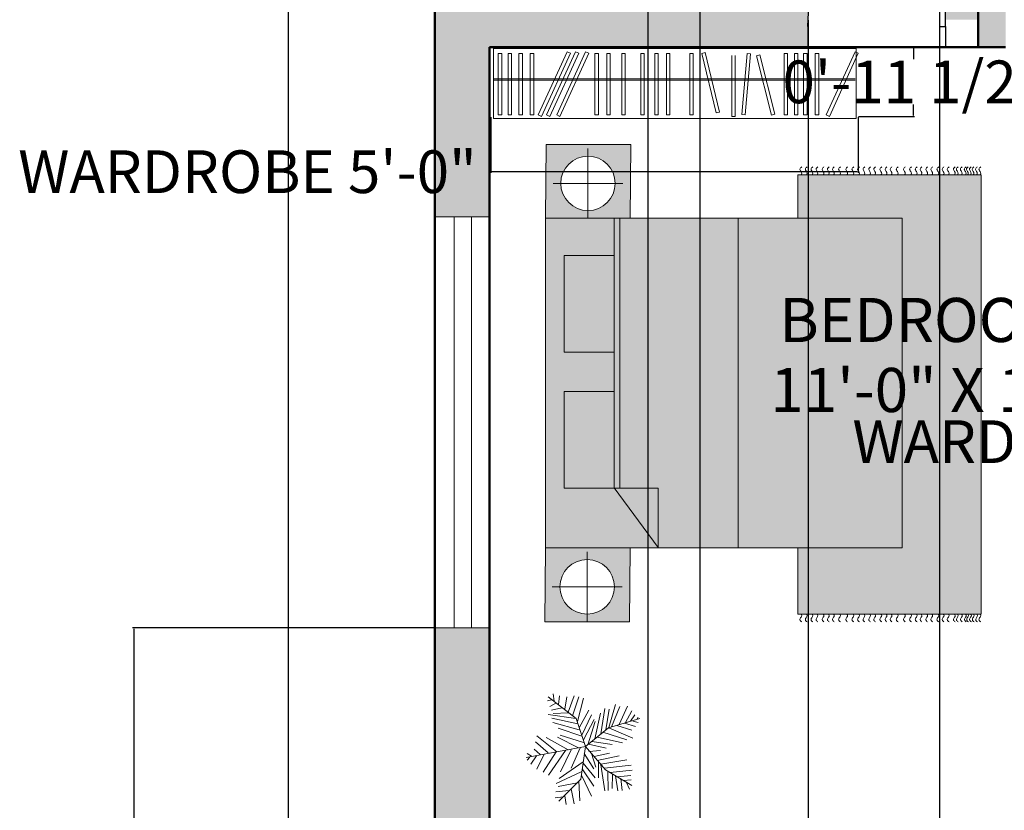
# Model space of a CAD drawing. Units: inches. Extents: x 2974 to 3443, y 2405 to 2963.
# Tile 10 of 13: x 2974 to 3136, y 2711 to 2840. Entities that reach past the tile are written whole.
import ezdxf

# ---------------------------------------------------------------- set-up
doc = ezdxf.new("R2010")
doc.units = ezdxf.units.IN
doc.header["$MEASUREMENT"] = 0
doc.layers.get('0').update_dxf_attribs({"color": 251})
for name, color, linetype, lineweight in [('A-ANNO-DIMS', 2, 'Continuous', 18), ('A-AREA-IDEN', 250, 'Continuous', 25), ('A-DOOR', 32, 'Continuous', 25), ('A-FLOR-PATT', 9, 'Continuous', 13), ('A-WALL-PATT', 252, 'Continuous', 13), ('closet', 32, 'Continuous', 20), ('furniture', 32, 'Continuous', 18), ('greenary', 106, 'Continuous', 13), ('walls', 250, 'Continuous', 50), ('windows', 159, 'Continuous', 20)]:
    doc.layers.add(name, color=color, linetype=linetype, lineweight=lineweight)
doc.layers.add('A-FURN-PATT', color=254, linetype='Continuous', lineweight=13, true_color=0xfeeab9)
doc.styles.get("Standard").update_dxf_attribs({"font": 'arial.ttf'})
doc.dimstyles.get("Standard").update_dxf_attribs({"dimtxt": 7, "dimasz": 0.18, "dimexe": 0.18, "dimexo": 0.0625, "dimgap": 0.09, "dimtad": 0, "dimtih": 1, "dimtoh": 1, "dimzin": 0, "dimdsep": 46, "dimlunit": 3, "dimtxsty": 'Standard', "dimcen": 0.09, "dimadec": 0, "dimazin": 0, "dimtfac": 1, "dimtofl": 0, "dimtmove": 0, "dimatfit": 3, "dimfxl": 1, "dimtolj": 1, "dimtzin": 0, "dimarcsym": 0})

# ---------------------------------------------------------------- blocks, each defined once
blk = doc.blocks.new('*U2')
for p, q in [((0, 0), (0, -6)), ((40, 0), (40, -6))]:
    blk.add_line(p, q)
blk.add_lwpolyline([(0, 0), (0, 40), (1.75, 40), (1.75, 0)], close=True)
blk.add_arc((0, 0), 40, 0, 90)
blk = doc.blocks.new('CARPET')
at = {"layer": 'furniture'}
for p, q in [((-51.53, -98.11), (-51.53, -55.12)), ((-51.53, -55.12), (-41.27, -55.12)), ((36, -55.12), (51.55, -55.12)), ((51.55, -55.12), (51.55, -98.11)), ((51.55, -98.11), (-51.53, -98.11))]:
    blk.add_line(p, q, dxfattribs=at)
for points, knots in [([(-53.37, -55.99), (-53.22, -55.8), (-52.9, -55.41), (-52.34, -55.8), (-51.89, -56.08), (-51.65, -55.91), (-51.53, -55.83)], [0, 0, 0, 0, 0.653278, 1.290138, 1.740457, 2.114451, 2.114451, 2.114451, 2.114451]), ([(-53.37, -57.26), (-53.22, -57.07), (-52.9, -56.67), (-52.34, -57.07), (-51.89, -57.35), (-51.65, -57.17), (-51.53, -57.1)], [0, 0, 0, 0, 0.653278, 1.290138, 1.740457, 2.114451, 2.114451, 2.114451, 2.114451]), ([(53.37, -55.99), (53.22, -55.8), (52.9, -55.41), (52.34, -55.8), (51.89, -56.08), (51.65, -55.91), (51.53, -55.83)], [0, 0, 0, 0, 0.653278, 1.290138, 1.740457, 2.114451, 2.114451, 2.114451, 2.114451]), ([(53.37, -57.26), (53.22, -57.07), (52.9, -56.67), (52.34, -57.07), (51.89, -57.35), (51.65, -57.17), (51.53, -57.1)], [0, 0, 0, 0, 0.653278, 1.290138, 1.740457, 2.114451, 2.114451, 2.114451, 2.114451]), ([(-53.37, -58.59), (-53.22, -58.4), (-52.9, -58.01), (-52.34, -58.4), (-51.89, -58.68), (-51.65, -58.5), (-51.53, -58.43)], [0, 0, 0, 0, 0.653278, 1.290138, 1.740457, 2.114451, 2.114451, 2.114451, 2.114451]), ([(-53.37, -59.78), (-53.22, -59.58), (-52.9, -59.19), (-52.34, -59.58), (-51.89, -59.86), (-51.65, -59.69), (-51.53, -59.61)], [0, 0, 0, 0, 0.653278, 1.290138, 1.740457, 2.114451, 2.114451, 2.114451, 2.114451]), ([(53.37, -58.59), (53.22, -58.4), (52.9, -58.01), (52.34, -58.4), (51.89, -58.68), (51.65, -58.5), (51.53, -58.43)], [0, 0, 0, 0, 0.653278, 1.290138, 1.740457, 2.114451, 2.114451, 2.114451, 2.114451]), ([(53.37, -59.78), (53.22, -59.58), (52.9, -59.19), (52.34, -59.58), (51.89, -59.86), (51.65, -59.69), (51.53, -59.61)], [0, 0, 0, 0, 0.653278, 1.290138, 1.740457, 2.114451, 2.114451, 2.114451, 2.114451]), ([(-53.37, -61.22), (-53.22, -61.02), (-52.9, -60.63), (-52.34, -61.02), (-51.89, -61.3), (-51.65, -61.13), (-51.53, -61.05)], [0, 0, 0, 0, 0.653278, 1.290138, 1.740457, 2.114451, 2.114451, 2.114451, 2.114451]), ([(-53.37, -62.44), (-53.22, -62.25), (-52.9, -61.86), (-52.34, -62.25), (-51.89, -62.53), (-51.65, -62.36), (-51.53, -62.28)], [0, 0, 0, 0, 0.653278, 1.290138, 1.740457, 2.114451, 2.114451, 2.114451, 2.114451]), ([(53.37, -61.22), (53.22, -61.02), (52.9, -60.63), (52.34, -61.02), (51.89, -61.3), (51.65, -61.13), (51.53, -61.05)], [0, 0, 0, 0, 0.653278, 1.290138, 1.740457, 2.114451, 2.114451, 2.114451, 2.114451]), ([(53.37, -62.44), (53.22, -62.25), (52.9, -61.86), (52.34, -62.25), (51.89, -62.53), (51.65, -62.36), (51.53, -62.28)], [0, 0, 0, 0, 0.653278, 1.290138, 1.740457, 2.114451, 2.114451, 2.114451, 2.114451]), ([(-53.37, -63.63), (-53.22, -63.43), (-52.9, -63.04), (-52.34, -63.43), (-51.89, -63.72), (-51.65, -63.54), (-51.53, -63.46)], [0, 0, 0, 0, 0.653278, 1.290138, 1.740457, 2.114451, 2.114451, 2.114451, 2.114451]), ([(-53.37, -65.07), (-53.22, -64.87), (-52.9, -64.48), (-52.34, -64.87), (-51.89, -65.15), (-51.65, -64.98), (-51.53, -64.9)], [0, 0, 0, 0, 0.653278, 1.290138, 1.740457, 2.114451, 2.114451, 2.114451, 2.114451]), ([(53.37, -63.63), (53.22, -63.43), (52.9, -63.04), (52.34, -63.43), (51.89, -63.72), (51.65, -63.54), (51.53, -63.46)], [0, 0, 0, 0, 0.653278, 1.290138, 1.740457, 2.114451, 2.114451, 2.114451, 2.114451]), ([(53.37, -65.07), (53.22, -64.87), (52.9, -64.48), (52.34, -64.87), (51.89, -65.15), (51.65, -64.98), (51.53, -64.9)], [0, 0, 0, 0, 0.653278, 1.290138, 1.740457, 2.114451, 2.114451, 2.114451, 2.114451]), ([(-53.37, -66.76), (-53.22, -66.56), (-52.9, -66.17), (-52.34, -66.56), (-51.89, -66.84), (-51.65, -66.67), (-51.53, -66.59)], [0, 0, 0, 0, 0.653278, 1.290138, 1.740457, 2.114451, 2.114451, 2.114451, 2.114451]), ([(53.37, -66.76), (53.22, -66.56), (52.9, -66.17), (52.34, -66.56), (51.89, -66.84), (51.65, -66.67), (51.53, -66.59)], [0, 0, 0, 0, 0.653278, 1.290138, 1.740457, 2.114451, 2.114451, 2.114451, 2.114451]), ([(-53.37, -68.2), (-53.22, -68), (-52.9, -67.61), (-52.34, -68), (-51.89, -68.28), (-51.65, -68.11), (-51.53, -68.03)], [0, 0, 0, 0, 0.653278, 1.290138, 1.740457, 2.114451, 2.114451, 2.114451, 2.114451]), ([(-53.37, -69.53), (-53.22, -69.33), (-52.9, -68.94), (-52.34, -69.33), (-51.89, -69.61), (-51.65, -69.44), (-51.53, -69.36)], [0, 0, 0, 0, 0.653278, 1.290138, 1.740457, 2.114451, 2.114451, 2.114451, 2.114451]), ([(53.37, -68.2), (53.22, -68), (52.9, -67.61), (52.34, -68), (51.89, -68.28), (51.65, -68.11), (51.53, -68.03)], [0, 0, 0, 0, 0.653278, 1.290138, 1.740457, 2.114451, 2.114451, 2.114451, 2.114451]), ([(53.37, -69.53), (53.22, -69.33), (52.9, -68.94), (52.34, -69.33), (51.89, -69.61), (51.65, -69.44), (51.53, -69.36)], [0, 0, 0, 0, 0.653278, 1.290138, 1.740457, 2.114451, 2.114451, 2.114451, 2.114451]), ([(-53.37, -70.79), (-53.22, -70.6), (-52.9, -70.21), (-52.34, -70.6), (-51.89, -70.88), (-51.65, -70.7), (-51.53, -70.63)], [0, 0, 0, 0, 0.653278, 1.290138, 1.740457, 2.114451, 2.114451, 2.114451, 2.114451]), ([(53.37, -70.79), (53.22, -70.6), (52.9, -70.21), (52.34, -70.6), (51.89, -70.88), (51.65, -70.7), (51.53, -70.63)], [0, 0, 0, 0, 0.653278, 1.290138, 1.740457, 2.114451, 2.114451, 2.114451, 2.114451]), ([(-53.37, -72.12), (-53.22, -71.93), (-52.9, -71.54), (-52.34, -71.93), (-51.89, -72.21), (-51.65, -72.04), (-51.53, -71.96)], [0, 0, 0, 0, 0.653278, 1.290138, 1.740457, 2.114451, 2.114451, 2.114451, 2.114451]), ([(-53.37, -73.31), (-53.22, -73.11), (-52.9, -72.72), (-52.34, -73.11), (-51.89, -73.4), (-51.65, -73.22), (-51.53, -73.14)], [0, 0, 0, 0, 0.653278, 1.290138, 1.740457, 2.114451, 2.114451, 2.114451, 2.114451]), ([(53.37, -72.12), (53.22, -71.93), (52.9, -71.54), (52.34, -71.93), (51.89, -72.21), (51.65, -72.04), (51.53, -71.96)], [0, 0, 0, 0, 0.653278, 1.290138, 1.740457, 2.114451, 2.114451, 2.114451, 2.114451]), ([(53.37, -73.31), (53.22, -73.11), (52.9, -72.72), (52.34, -73.11), (51.89, -73.4), (51.65, -73.22), (51.53, -73.14)], [0, 0, 0, 0, 0.653278, 1.290138, 1.740457, 2.114451, 2.114451, 2.114451, 2.114451]), ([(-53.37, -74.75), (-53.22, -74.55), (-52.9, -74.16), (-52.34, -74.55), (-51.89, -74.83), (-51.65, -74.66), (-51.53, -74.58)], [0, 0, 0, 0, 0.653278, 1.290138, 1.740457, 2.114451, 2.114451, 2.114451, 2.114451]), ([(-53.37, -75.98), (-53.22, -75.78), (-52.9, -75.39), (-52.34, -75.78), (-51.89, -76.06), (-51.65, -75.89), (-51.53, -75.81)], [0, 0, 0, 0, 0.653278, 1.290138, 1.740457, 2.114451, 2.114451, 2.114451, 2.114451]), ([(53.37, -74.75), (53.22, -74.55), (52.9, -74.16), (52.34, -74.55), (51.89, -74.83), (51.65, -74.66), (51.53, -74.58)], [0, 0, 0, 0, 0.653278, 1.290138, 1.740457, 2.114451, 2.114451, 2.114451, 2.114451]), ([(53.37, -75.98), (53.22, -75.78), (52.9, -75.39), (52.34, -75.78), (51.89, -76.06), (51.65, -75.89), (51.53, -75.81)], [0, 0, 0, 0, 0.653278, 1.290138, 1.740457, 2.114451, 2.114451, 2.114451, 2.114451]), ([(-53.37, -77.16), (-53.22, -76.96), (-52.9, -76.57), (-52.34, -76.96), (-51.89, -77.25), (-51.65, -77.07), (-51.53, -76.99)], [0, 0, 0, 0, 0.653278, 1.290138, 1.740457, 2.114451, 2.114451, 2.114451, 2.114451]), ([(-53.37, -78.6), (-53.22, -78.4), (-52.9, -78.01), (-52.34, -78.4), (-51.89, -78.68), (-51.65, -78.51), (-51.53, -78.43)], [0, 0, 0, 0, 0.653278, 1.290138, 1.740457, 2.114451, 2.114451, 2.114451, 2.114451]), ([(53.37, -77.16), (53.22, -76.96), (52.9, -76.57), (52.34, -76.96), (51.89, -77.25), (51.65, -77.07), (51.53, -76.99)], [0, 0, 0, 0, 0.653278, 1.290138, 1.740457, 2.114451, 2.114451, 2.114451, 2.114451]), ([(53.37, -78.6), (53.22, -78.4), (52.9, -78.01), (52.34, -78.4), (51.89, -78.68), (51.65, -78.51), (51.53, -78.43)], [0, 0, 0, 0, 0.653278, 1.290138, 1.740457, 2.114451, 2.114451, 2.114451, 2.114451]), ([(-53.37, -80.29), (-53.22, -80.09), (-52.9, -79.7), (-52.34, -80.09), (-51.89, -80.37), (-51.65, -80.2), (-51.53, -80.12)], [0, 0, 0, 0, 0.653278, 1.290138, 1.740457, 2.114451, 2.114451, 2.114451, 2.114451]), ([(53.37, -80.29), (53.22, -80.09), (52.9, -79.7), (52.34, -80.09), (51.89, -80.37), (51.65, -80.2), (51.53, -80.12)], [0, 0, 0, 0, 0.653278, 1.290138, 1.740457, 2.114451, 2.114451, 2.114451, 2.114451]), ([(-53.37, -81.73), (-53.22, -81.53), (-52.9, -81.14), (-52.34, -81.53), (-51.89, -81.81), (-51.65, -81.64), (-51.53, -81.56)], [0, 0, 0, 0, 0.653278, 1.290138, 1.740457, 2.114451, 2.114451, 2.114451, 2.114451]), ([(-53.37, -83.06), (-53.22, -82.86), (-52.9, -82.47), (-52.34, -82.86), (-51.89, -83.14), (-51.65, -82.97), (-51.53, -82.89)], [0, 0, 0, 0, 0.653278, 1.290138, 1.740457, 2.114451, 2.114451, 2.114451, 2.114451]), ([(53.37, -81.73), (53.22, -81.53), (52.9, -81.14), (52.34, -81.53), (51.89, -81.81), (51.65, -81.64), (51.53, -81.56)], [0, 0, 0, 0, 0.653278, 1.290138, 1.740457, 2.114451, 2.114451, 2.114451, 2.114451]), ([(53.37, -83.06), (53.22, -82.86), (52.9, -82.47), (52.34, -82.86), (51.89, -83.14), (51.65, -82.97), (51.53, -82.89)], [0, 0, 0, 0, 0.653278, 1.290138, 1.740457, 2.114451, 2.114451, 2.114451, 2.114451]), ([(-53.37, -84.18), (-53.22, -83.99), (-52.9, -83.6), (-52.34, -83.99), (-51.89, -84.27), (-51.65, -84.09), (-51.53, -84.02)], [0, 0, 0, 0, 0.653278, 1.290138, 1.740457, 2.114451, 2.114451, 2.114451, 2.114451]), ([(-53.37, -85.51), (-53.22, -85.32), (-52.9, -84.93), (-52.34, -85.32), (-51.89, -85.6), (-51.65, -85.42), (-51.53, -85.35)], [0, 0, 0, 0, 0.653278, 1.290138, 1.740457, 2.114451, 2.114451, 2.114451, 2.114451]), ([(53.37, -84.18), (53.22, -83.99), (52.9, -83.6), (52.34, -83.99), (51.89, -84.27), (51.65, -84.09), (51.53, -84.02)], [0, 0, 0, 0, 0.653278, 1.290138, 1.740457, 2.114451, 2.114451, 2.114451, 2.114451]), ([(53.37, -85.51), (53.22, -85.32), (52.9, -84.93), (52.34, -85.32), (51.89, -85.6), (51.65, -85.42), (51.53, -85.35)], [0, 0, 0, 0, 0.653278, 1.290138, 1.740457, 2.114451, 2.114451, 2.114451, 2.114451]), ([(-53.37, -86.7), (-53.22, -86.5), (-52.9, -86.11), (-52.34, -86.5), (-51.89, -86.78), (-51.65, -86.61), (-51.53, -86.53)], [0, 0, 0, 0, 0.653278, 1.290138, 1.740457, 2.114451, 2.114451, 2.114451, 2.114451]), ([(-53.37, -88.14), (-53.22, -87.94), (-52.9, -87.55), (-52.34, -87.94), (-51.89, -88.22), (-51.65, -88.05), (-51.53, -87.97)], [0, 0, 0, 0, 0.653278, 1.290138, 1.740457, 2.114451, 2.114451, 2.114451, 2.114451]), ([(53.37, -86.7), (53.22, -86.5), (52.9, -86.11), (52.34, -86.5), (51.89, -86.78), (51.65, -86.61), (51.53, -86.53)], [0, 0, 0, 0, 0.653278, 1.290138, 1.740457, 2.114451, 2.114451, 2.114451, 2.114451]), ([(53.37, -88.14), (53.22, -87.94), (52.9, -87.55), (52.34, -87.94), (51.89, -88.22), (51.65, -88.05), (51.53, -87.97)], [0, 0, 0, 0, 0.653278, 1.290138, 1.740457, 2.114451, 2.114451, 2.114451, 2.114451]), ([(-53.37, -89.36), (-53.22, -89.17), (-52.9, -88.78), (-52.34, -89.17), (-51.89, -89.45), (-51.65, -89.28), (-51.53, -89.2)], [0, 0, 0, 0, 0.653278, 1.290138, 1.740457, 2.114451, 2.114451, 2.114451, 2.114451]), ([(53.37, -89.36), (53.22, -89.17), (52.9, -88.78), (52.34, -89.17), (51.89, -89.45), (51.65, -89.28), (51.53, -89.2)], [0, 0, 0, 0, 0.653278, 1.290138, 1.740457, 2.114451, 2.114451, 2.114451, 2.114451]), ([(-53.37, -90.55), (-53.22, -90.35), (-52.9, -89.96), (-52.34, -90.35), (-51.89, -90.64), (-51.65, -90.46), (-51.53, -90.38)], [0, 0, 0, 0, 0.653278, 1.290138, 1.740457, 2.114451, 2.114451, 2.114451, 2.114451]), ([(-53.37, -91.99), (-53.22, -91.79), (-52.9, -91.4), (-52.34, -91.79), (-51.89, -92.07), (-51.65, -91.9), (-51.53, -91.82)], [0, 0, 0, 0, 0.653278, 1.290138, 1.740457, 2.114451, 2.114451, 2.114451, 2.114451]), ([(-53.37, -92.69), (-53.22, -92.48), (-52.9, -92.08), (-52.35, -92.49), (-51.89, -92.77), (-51.65, -92.6), (-51.53, -92.52)], [0, 0, 0, 0, 0.663904, 1.307406, 1.757725, 2.131719, 2.131719, 2.131719, 2.131719]), ([(53.37, -90.55), (53.22, -90.35), (52.9, -89.96), (52.34, -90.35), (51.9, -90.63), (51.66, -90.47), (51.55, -90.4)], [0, 0, 0, 0, 0.653278, 1.290138, 1.740457, 2.0926, 2.0926, 2.0926, 2.0926]), ([(53.37, -91.99), (53.22, -91.79), (52.9, -91.4), (52.34, -91.79), (51.9, -92.07), (51.66, -91.91), (51.55, -91.83)], [0, 0, 0, 0, 0.653278, 1.290138, 1.740457, 2.0926, 2.0926, 2.0926, 2.0926]), ([(53.37, -92.69), (53.22, -92.49), (52.9, -92.09), (52.34, -92.49), (51.9, -92.77), (51.66, -92.61), (51.55, -92.53)], [0, 0, 0, 0, 0.656792, 1.295826, 1.746145, 2.098292, 2.098292, 2.098292, 2.098292]), ([(-53.37, -93.61), (-53.22, -93.42), (-52.9, -93.03), (-52.34, -93.42), (-51.89, -93.7), (-51.65, -93.52), (-51.53, -93.45)], [0, 0, 0, 0, 0.653278, 1.290138, 1.740457, 2.114451, 2.114451, 2.114451, 2.114451]), ([(-53.37, -94.55), (-53.22, -94.35), (-52.9, -93.96), (-52.34, -94.35), (-51.89, -94.63), (-51.65, -94.46), (-51.53, -94.38)], [0, 0, 0, 0, 0.653278, 1.290138, 1.740457, 2.114451, 2.114451, 2.114451, 2.114451]), ([(-53.37, -95.05), (-53.22, -94.85), (-52.9, -94.46), (-52.34, -94.85), (-51.89, -95.14), (-51.65, -94.96), (-51.53, -94.88)], [0, 0, 0, 0, 0.653278, 1.290138, 1.740457, 2.114451, 2.114451, 2.114451, 2.114451]), ([(53.37, -93.66), (53.22, -93.46), (52.9, -93.07), (52.34, -93.46), (51.9, -93.74), (51.66, -93.58), (51.55, -93.5)], [0, 0, 0, 0, 0.653278, 1.290138, 1.740457, 2.0926, 2.0926, 2.0926, 2.0926]), ([(53.37, -94.59), (53.22, -94.4), (52.9, -94.01), (52.34, -94.4), (51.9, -94.68), (51.66, -94.51), (51.55, -94.44)], [0, 0, 0, 0, 0.653278, 1.290138, 1.740457, 2.0926, 2.0926, 2.0926, 2.0926]), ([(53.37, -95.1), (53.22, -94.9), (52.9, -94.51), (52.34, -94.9), (51.9, -95.18), (51.66, -95.02), (51.55, -94.94)], [0, 0, 0, 0, 0.653278, 1.290138, 1.740457, 2.0926, 2.0926, 2.0926, 2.0926]), ([(-53.37, -95.73), (-53.22, -95.54), (-52.9, -95.15), (-52.34, -95.54), (-51.89, -95.82), (-51.65, -95.65), (-51.53, -95.57)], [0, 0, 0, 0, 0.653278, 1.290138, 1.740457, 2.114451, 2.114451, 2.114451, 2.114451]), ([(-53.37, -96.38), (-53.22, -96.18), (-52.9, -95.79), (-52.34, -96.18), (-51.89, -96.47), (-51.65, -96.29), (-51.53, -96.21)], [0, 0, 0, 0, 0.653278, 1.290138, 1.740457, 2.114451, 2.114451, 2.114451, 2.114451]), ([(-53.37, -97.17), (-53.22, -96.98), (-52.9, -96.59), (-52.34, -96.98), (-51.89, -97.26), (-51.65, -97.08), (-51.53, -97.01)], [0, 0, 0, 0, 0.653278, 1.290138, 1.740457, 2.114451, 2.114451, 2.114451, 2.114451]), ([(53.37, -95.78), (53.22, -95.58), (52.9, -95.19), (52.34, -95.58), (51.89, -95.86), (51.65, -95.69), (51.53, -95.61)], [0, 0, 0, 0, 0.653278, 1.290138, 1.740457, 2.114451, 2.114451, 2.114451, 2.114451]), ([(53.37, -96.43), (53.22, -96.23), (52.9, -95.84), (52.34, -96.23), (51.89, -96.51), (51.65, -96.34), (51.53, -96.26)], [0, 0, 0, 0, 0.653278, 1.290138, 1.740457, 2.114451, 2.114451, 2.114451, 2.114451]), ([(53.37, -97.22), (53.22, -97.02), (52.9, -96.63), (52.34, -97.02), (51.89, -97.3), (51.65, -97.13), (51.53, -97.05)], [0, 0, 0, 0, 0.653278, 1.290138, 1.740457, 2.114451, 2.114451, 2.114451, 2.114451]), ([(-53.37, -97.99), (-53.22, -97.79), (-52.9, -97.4), (-52.34, -97.79), (-51.89, -98.08), (-51.65, -97.9), (-51.53, -97.82)], [0, 0, 0, 0, 0.653278, 1.290138, 1.740457, 2.114451, 2.114451, 2.114451, 2.114451]), ([(53.37, -97.99), (53.22, -97.79), (52.9, -97.4), (52.34, -97.79), (51.89, -98.08), (51.65, -97.9), (51.53, -97.82)], [0, 0, 0, 0, 0.653278, 1.290138, 1.740457, 2.114451, 2.114451, 2.114451, 2.114451])]:
    blk.add_open_spline(points, degree=3, knots=knots, dxfattribs=at)
blk = doc.blocks.new('A$C58D270C6')
at = {"layer": 'furniture'}
for p, q in [((9.09, 124.13), (9.09, 108.87)), ((1.46, 116.5), (16.73, 116.5)), ((14.97, 94.84), (24.62, 107.92)), ((24.62, 94.93), (24.62, 107.92)), ((42.08, 108), (42.08, 36)), ((14.97, 94.93), (24.62, 94.93)), ((14.97, 94.84), (14.97, 36)), ((16.22, 94.93), (16.22, 36)), ((9.25, 36), (9.25, 20.74)), ((1.62, 28.37), (16.88, 28.37))]:
    blk.add_line(p, q, dxfattribs=at)
for points in [[(18.5, 108), (18.34, 124.13), (-0.16, 124.13), (0, 108)], [(0, 108), (77.91, 108), (77.91, 36), (0, 36)], [(4.09, 94.93), (14.97, 94.93), (14.97, 73.83), (4.09, 73.83)], [(4.09, 65.23), (14.97, 65.23), (14.97, 44.13), (4.09, 44.13)], [(18.65, 19.87), (18.5, 36), (0, 36), (0.16, 19.87)]]:
    blk.add_lwpolyline(points, close=True, dxfattribs=at)
for centre in [(9.09, 116.5), (9.25, 28.37)]:
    blk.add_circle(centre, 5.95, dxfattribs=at)
at = {"layer": 'furniture', "xscale": 0.9312884925094044, "yscale": 0.9312884925094044, "zscale": 0.9312884925094044, "rotation": 90}
blk.add_blockref('CARPET', (3.79, 74.47), dxfattribs=at)
blk = doc.blocks.new('closet')
at = {"layer": 'closet'}
for p, q in [((-0.71, -5.58), (5.59, 8.19)), ((-0.23, 7.39), (-0.23, -6.57)), ((6.27, 7.88), (-0.04, -5.89)), ((5.59, 8.19), (6.27, 7.88)), ((7.92, 7.84), (8.68, 7.84)), ((7.92, 7.84), (7.92, -5.51)), ((8.68, 7.84), (8.68, -5.51)), ((10.44, 7.84), (11.2, 7.84)), ((10.44, 7.84), (10.44, -5.51)), ((11.2, 7.84), (11.2, -5.51)), ((12.45, 7.84), (13.21, 7.84)), ((12.45, 7.84), (12.45, -5.51)), ((13.21, 7.84), (13.21, -5.51)), ((14.71, 7.84), (15.47, 7.84)), ((14.71, 7.84), (14.71, -5.51)), ((15.47, 7.84), (15.47, -5.51)), ((17.44, 7.75), (18.17, 7.93)), ((17.44, 7.75), (20.73, -5.2)), ((18.17, 7.93), (21.46, -5.01)), ((23.92, 7.84), (22.75, -5.46)), ((24.67, 7.78), (23.51, -5.53)), ((23.92, 7.84), (24.67, 7.78)), ((26.09, 8.25), (26.09, -5.1)), ((26.84, 8.25), (26.84, -5.1)), ((29.49, 7.29), (32.64, -5.69)), ((30.22, 7.46), (33.37, -5.51)), ((35.23, 7.84), (35.23, -5.51)), ((35.99, 7.84), (35.99, -5.51)), ((40.33, 7.84), (40.33, -5.51)), ((41.08, 7.84), (41.08, -5.51)), ((42.85, 7.84), (42.85, -5.51)), ((43.61, 7.84), (43.61, -5.51)), ((45.9, 7.84), (45.9, -5.51)), ((46.65, 7.84), (46.65, -5.51)), ((50.07, 7.84), (50.07, -5.51)), ((50.82, 7.84), (50.82, -5.51)), ((53.32, 7.84), (53.32, -5.51)), ((54.08, 7.84), (54.08, -5.51)), ((55.9, 7.84), (55.9, -5.51)), ((56.65, 7.84), (56.65, -5.51)), ((57.99, -5.58), (64.3, 8.19)), ((64.97, 7.88), (58.67, -5.89)), ((60.19, -5.58), (66.49, 8.19)), ((67.17, 7.88), (60.87, -5.89)), ((62, -5.58), (68.3, 8.19)), ((68.98, 7.88), (62.67, -5.89)), ((69.96, 7.84), (69.96, -5.51)), ((70.72, 7.84), (70.72, -5.51)), ((72.43, 7.84), (72.43, -5.51)), ((73.19, 7.84), (73.19, -5.51)), ((74.82, 7.84), (74.82, -5.51)), ((75.57, 7.84), (75.57, -5.51)), ((76.94, 7.84), (76.94, -5.51)), ((77.69, 7.84), (77.69, -5.51)), ((56.23, 0.33), (0, 0.33)), ((56.2, 0), (0, 0)), ((56.2, 0), (78.76, 0)), ((56.23, 0.33), (78.76, 0.33)), ((-0.04, -5.89), (-0.71, -5.58)), ((21.46, -5.01), (20.73, -5.2)), ((23.51, -5.53), (22.75, -5.46)), ((33.37, -5.51), (32.64, -5.69)), ((35.99, -5.51), (35.23, -5.51)), ((41.08, -5.51), (40.33, -5.51)), ((43.61, -5.51), (42.85, -5.51)), ((46.65, -5.51), (45.9, -5.51)), ((50.82, -5.51), (50.07, -5.51)), ((54.08, -5.51), (53.32, -5.51)), ((56.65, -5.51), (55.9, -5.51)), ((58.67, -5.89), (57.99, -5.58)), ((60.87, -5.89), (60.19, -5.58)), ((62.67, -5.89), (62, -5.58)), ((70.72, -5.51), (69.96, -5.51)), ((73.19, -5.51), (72.43, -5.51)), ((75.57, -5.51), (74.82, -5.51)), ((77.69, -5.51), (76.94, -5.51))]:
    blk.add_line(p, q, dxfattribs=at)
blk = doc.blocks.new('rotated closet')
at = {"layer": 'closet'}
for p, q in [((26.32, 0.86), (27.07, 0.86)), ((29.72, -0.11), (30.45, 0.07)), ((35.46, 0.45), (36.22, 0.45)), ((40.56, 0.45), (41.31, 0.45)), ((43.08, 0.45), (43.84, 0.45)), ((46.13, 0.45), (46.88, 0.45)), ((50.3, 0.45), (51.05, 0.45)), ((53.56, 0.45), (54.31, 0.45)), ((56.13, 0.45), (56.88, 0.45)), ((64.53, 0.8), (65.2, 0.49)), ((66.72, 0.8), (67.4, 0.49)), ((68.53, 0.8), (69.21, 0.49)), ((70.19, 0.45), (70.95, 0.45)), ((72.66, 0.45), (73.42, 0.45)), ((75.05, 0.45), (75.81, 0.45)), ((77.17, 0.45), (77.92, 0.45)), ((78.99, 0), (78.99, -13.96)), ((-0.46, -14.27), (79.54, -14.27)), ((0, -13.96), (78.99, -13.96)), ((8.91, -12.91), (8.15, -12.91)), ((11.43, -12.91), (10.67, -12.91)), ((13.44, -12.91), (12.68, -12.91)), ((15.7, -12.91), (14.94, -12.91))]:
    blk.add_line(p, q, dxfattribs=at)
blk.add_blockref('closet', (0.23, -7.39), dxfattribs=at)
blk = doc.blocks.new('*U13')
for p, q in [((0, 0), (-10.5, 57)), ((-8.737, 47.138), (-17.069, 52.711)), ((-10.186, 53.64), (-13.084, 55.962)), ((-9.099, 51.782), (-6.563, 55.962)), ((-7.65, 43.423), (-2.578, 49.46)), ((-5.839, 35.992), (4.667, 48.067)), ((-5.114, 28.097), (-24.676, 40.636)), ((-7.288, 39.707), (-21.778, 46.673)), ((-5.114, 27.632), (10.463, 46.673)), ((-48.585, 21.131), (-49.309, 29.026)), ((-43.513, 28.561), (-42.427, 15.558)), ((-3.665, 19.273), (-27.574, 35.527)), ((-2.941, 16.486), (8.652, 37.85)), ((16.259, 5.805), (23.142, 31.348)), ((22.055, 7.198), (27.489, 32.277)), ((27, 9), (48, 36)), ((27.127, 9.056), (31.112, 35.992)), ((31.836, 30.883), (32.561, 16.486)), ((35.096, 32.741), (37.27, 22.524)), ((38.719, 34.134), (41.979, 28.561)), ((43.791, 29.954), (51.036, 30.883)), ((44.153, 36.456), (45.239, 32.741)), ((-47.498, 19.737), (-55.83, 18.344)), ((-31.5, 4.5), (-52.5, 25.5)), ((-38.442, 26.239), (-34.819, 7.663)), ((-35.544, 28.097), (-24.314, 3.947)), ((-14.533, 2.09), (-30.834, 25.31)), ((-24.314, 23.917), (-2.941, 13.7)), ((-1.129, 6.734), (9.014, 26.704)), ((3.942, 1.625), (11.187, 24.381)), ((10.101, 3.483), (17.708, 26.239)), ((36.183, 19.737), (48.137, 17.88)), ((40.53, 25.775), (48.862, 24.846)), ((-40.615, 13.7), (-55.105, 10.913)), ((-20.691, 13.7), (-1.129, 4.876)), ((29.662, 12.307), (48.137, 6.269)), ((33.285, 16.486), (48.862, 10.913)), ((-33.37, 6.269), (-52.207, 5.34)), ((-28.299, 3.483), (-47.86, -5.805)), ((-21.416, 3.018), (-38.079, -8.128)), ((0, 0), (-31.5, 4.5)), ((-15.982, 2.09), (-30.11, -9.521)), ((0, 0), (-22.5, -19.5)), ((-6.563, 1.161), (-21.416, -8.128)), ((0, 0), (27, 9)), ((0, 0), (18, -22.5)), ((6.478, 1.625), (26.04, -8.592)), ((11.187, 3.483), (30.749, -5.805)), ((18.07, 5.805), (35.096, -3.483)), ((24.229, 7.663), (46.688, 1.625)), ((-6.563, -5.805), (-19.967, -9.985)), ((-9.461, -8.592), (-6.201, -23.453)), ((-4.752, -3.483), (-3.665, -14.629)), ((2.493, -3.019), (-1.491, -20.202)), ((1.769, -2.555), (24.229, -9.521)), ((5.029, -6.27), (2.131, -25.775)), ((7.565, -9.056), (32.198, -14.629)), ((-17.431, -15.094), (-42.789, -18.809)), ((-15.257, -12.772), (-30.11, -12.772)), ((-20.691, -18.345), (-17.793, -44.352)), ((-17.069, -15.094), (-12.721, -40.172)), ((-13.446, -11.378), (-8.737, -32.741)), ((9.014, -11.378), (3.58, -35.992)), ((14.085, -16.951), (6.478, -40.172)), ((12.274, -15.094), (36.907, -18.809)), ((-24.314, -21.596), (-42.427, -22.06)), ((-26.849, -26.24), (-40.253, -25.775)), ((-22.5, -19.5), (-37.5, -45)), ((-25.038, -23.918), (-22.865, -45.281)), ((18.07, -22.524), (8.289, -45.745)), ((16.259, -19.738), (36.183, -22.989)), ((18, -22.5), (27, -52.5)), ((18.433, -22.524), (40.53, -29.026)), ((19.157, -25.311), (38.719, -33.206)), ((-28.299, -29.026), (-42.789, -31.348)), ((-30.834, -34.135), (-42.427, -35.528)), ((-32.646, -36.921), (-31.921, -44.352)), ((-29.023, -30.884), (-27.936, -43.887)), ((20.244, -30.419), (15.897, -44.816)), ((22.78, -37.85), (19.519, -48.532)), ((21.331, -32.741), (39.081, -40.636)), ((-34.457, -39.708), (-40.978, -42.494)), ((22.78, -38.314), (34.372, -44.816)), ((24.591, -45.745), (23.142, -50.854)), ((24.591, -43.423), (30.749, -47.603)), ((26.764, -49.925), (28.213, -50.854))]:
    blk.add_line(p, q)
blk = doc.blocks.new('*D20')
at = {"layer": 'A-ANNO-DIMS', "color": 0, "lineweight": -2, "transparency": 16777216}
for p, q in [((3018.41, 2903.19), (3018.14, 2903.19)), ((3018.32, 2903.01), (3018.32, 2690.85)), ((3018.32, 2471.37), (3018.32, 2683.52)), ((3018.41, 2471.19), (3018.14, 2471.19))]:
    blk.add_line(p, q, dxfattribs=at)
at = {"layer": 'A-ANNO-DIMS', "color": 0, "transparency": 16777216}
for points in [[(3018.29, 2903.01), (3018.35, 2903.01), (3018.32, 2903.19)], [(3018.29, 2471.37), (3018.35, 2471.37), (3018.32, 2471.19)]]:
    blk.add_solid(points, dxfattribs=at)
at = {"layer": 'Defpoints', "color": 0, "transparency": 16777216}
for p in [(3018.47, 2903.19), (3018.32, 2471.19), (3018.47, 2471.19)]:
    blk.add_point(p, dxfattribs=at)
at = {"layer": 'A-ANNO-DIMS', "color": 0, "transparency": 16777216, "insert": (3018.32, 2687.19), "char_height": 7, "attachment_point": 5}
blk.add_mtext("\\A1;36'", dxfattribs=at)
blk = doc.blocks.new('WIN-67IN')
for p, q in [((0, 0), (9, 0)), ((0, -67.29), (0, 0)), ((0, 0), (3.19, 0)), ((3.19, 0), (3.19, -67.29)), ((6.02, -67.29), (6.02, 0)), ((9, 0), (9, -67.29)), ((9, -67.29), (0, -67.29)), ((3.19, -67.29), (6.02, -67.29))]:
    blk.add_line(p, q)
blk = doc.blocks.new('*D27')
at = {"layer": 'A-ANNO-DIMS', "color": 0, "lineweight": -2, "transparency": 16777216}
for p, q in [((3051.53, 2824.24), (3051.53, 2815.1)), ((3111.71, 2824.24), (3111.71, 2815.1)), ((3051.53, 2815.28), (3051.35, 2815.28)), ((3111.53, 2815.28), (3051.71, 2815.28))]:
    blk.add_line(p, q, dxfattribs=at)
at = {"layer": 'A-ANNO-DIMS', "color": 0, "transparency": 16777216}
for points in [[(3051.71, 2815.31), (3051.71, 2815.25), (3051.53, 2815.28)], [(3111.53, 2815.31), (3111.53, 2815.25), (3111.71, 2815.28)]]:
    blk.add_solid(points, dxfattribs=at)
at = {"layer": 'Defpoints', "color": 0, "transparency": 16777216}
for p in [(3051.53, 2824.31), (3111.71, 2824.31), (3051.53, 2815.28)]:
    blk.add_point(p, dxfattribs=at)
at = {"layer": 'A-ANNO-DIMS', "color": 0, "transparency": 16777216, "insert": (3011.66, 2815.28), "char_height": 7, "attachment_point": 5}
blk.add_mtext('\\A1;WARDROBE 5\'-0"', dxfattribs=at)
blk = doc.blocks.new('*D28')
at = {"layer": 'A-ANNO-DIMS', "color": 0, "lineweight": -2, "transparency": 16777216}
for p, q in [((3111.77, 2835.69), (3120.92, 2835.69)), ((3120.74, 2835.51), (3120.74, 2833.71)), ((3120.74, 2824.49), (3120.74, 2826.29)), ((3111.77, 2824.31), (3120.92, 2824.31))]:
    blk.add_line(p, q, dxfattribs=at)
at = {"layer": 'A-ANNO-DIMS', "color": 0, "transparency": 16777216}
for points in [[(3120.71, 2835.51), (3120.77, 2835.51), (3120.74, 2835.69)], [(3120.71, 2824.49), (3120.77, 2824.49), (3120.74, 2824.31)]]:
    blk.add_solid(points, dxfattribs=at)
at = {"layer": 'Defpoints', "color": 0, "transparency": 16777216}
for p in [(3111.71, 2835.69), (3111.71, 2824.31), (3120.74, 2824.31)]:
    blk.add_point(p, dxfattribs=at)
at = {"layer": 'A-ANNO-DIMS', "color": 0, "transparency": 16777216, "insert": (3120.74, 2830), "char_height": 7, "attachment_point": 5}
blk.add_mtext('\\A1;0\'-11 1/2"', dxfattribs=at)
blk = doc.blocks.new('*D29')
at = {"layer": 'A-ANNO-DIMS', "color": 0, "lineweight": -2, "transparency": 16777216}
for p, q in [((3188.17, 2771.05), (3187.99, 2771.05)), ((3188.17, 2764.54), (3188.17, 2771.23)), ((3231.81, 2771.05), (3188.35, 2771.05)), ((3231.99, 2764.54), (3231.99, 2771.23))]:
    blk.add_line(p, q, dxfattribs=at)
at = {"layer": 'A-ANNO-DIMS', "color": 0, "transparency": 16777216}
for points in [[(3188.35, 2771.08), (3188.35, 2771.02), (3188.17, 2771.05)], [(3231.81, 2771.08), (3231.81, 2771.02), (3231.99, 2771.05)]]:
    blk.add_solid(points, dxfattribs=at)
at = {"layer": 'Defpoints', "color": 0, "transparency": 16777216}
for p in [(3188.17, 2771.05), (3188.17, 2764.48), (3231.99, 2764.48)]:
    blk.add_point(p, dxfattribs=at)
at = {"layer": 'A-ANNO-DIMS', "color": 0, "transparency": 16777216, "insert": (3148.3, 2771.05), "char_height": 7, "attachment_point": 5}
blk.add_mtext('\\A1;WARDROBE 3\'-8"', dxfattribs=at)
blk = doc.blocks.new('*D55')
at = {"layer": 'A-ANNO-DIMS', "color": 0, "lineweight": -2, "transparency": 16777216}
for p, q in [((3042.26, 2740.57), (2992.84, 2740.57)), ((2993.02, 2740.39), (2993.02, 2699.61)), ((2993.02, 2651.41), (2993.02, 2692.19)), ((3042.26, 2651.23), (2992.84, 2651.23))]:
    blk.add_line(p, q, dxfattribs=at)
at = {"layer": 'A-ANNO-DIMS', "color": 0, "transparency": 16777216}
for points in [[(2992.99, 2740.39), (2993.05, 2740.39), (2993.02, 2740.57)], [(2992.99, 2651.41), (2993.05, 2651.41), (2993.02, 2651.23)]]:
    blk.add_solid(points, dxfattribs=at)
at = {"layer": 'Defpoints', "color": 0, "transparency": 16777216}
for p in [(3042.33, 2740.57), (2993.02, 2651.23), (3042.33, 2651.23)]:
    blk.add_point(p, dxfattribs=at)
at = {"layer": 'A-ANNO-DIMS', "color": 0, "transparency": 16777216, "insert": (2993.02, 2695.9), "char_height": 7, "attachment_point": 5}
blk.add_mtext('\\A1;7\'-5 1/2"', dxfattribs=at)
blk = doc.blocks.new('*D64')
at = {"layer": 'A-ANNO-DIMS', "color": 0, "lineweight": -2, "transparency": 16777216}
for p, q in [((3103.48, 2840.13), (3103.48, 2414.92)), ((3124.99, 2840.13), (3124.99, 2414.92)), ((3103.66, 2415.1), (3124.81, 2415.1)), ((3124.99, 2415.1), (3125.17, 2415.1))]:
    blk.add_line(p, q, dxfattribs=at)
at = {"layer": 'A-ANNO-DIMS', "color": 0, "transparency": 16777216}
for points in [[(3103.66, 2415.13), (3103.66, 2415.07), (3103.48, 2415.1)], [(3124.81, 2415.13), (3124.81, 2415.07), (3124.99, 2415.1)]]:
    blk.add_solid(points, dxfattribs=at)
at = {"layer": 'Defpoints', "color": 0, "transparency": 16777216}
for p in [(3103.48, 2840.19), (3124.99, 2840.19), (3124.99, 2415.1)]:
    blk.add_point(p, dxfattribs=at)
at = {"layer": 'A-ANNO-DIMS', "color": 0, "transparency": 16777216, "insert": (3142.39, 2415.1), "char_height": 7, "attachment_point": 5}
blk.add_mtext('\\A1;1\'-9 1/2"', dxfattribs=at)
blk = doc.blocks.new('*D68')
at = {"layer": 'A-ANNO-DIMS', "color": 0, "lineweight": -2, "transparency": 16777216}
for p, q in [((3077.27, 2480.25), (3077.27, 2952.68)), ((3077.45, 2952.5), (3085.63, 2952.5)), ((3085.81, 2480.25), (3085.81, 2952.68)), ((3085.81, 2952.5), (3085.99, 2952.5))]:
    blk.add_line(p, q, dxfattribs=at)
at = {"layer": 'A-ANNO-DIMS', "color": 0, "transparency": 16777216}
for points in [[(3077.45, 2952.53), (3077.45, 2952.47), (3077.27, 2952.5)], [(3085.63, 2952.53), (3085.63, 2952.47), (3085.81, 2952.5)]]:
    blk.add_solid(points, dxfattribs=at)
at = {"layer": 'Defpoints', "color": 0, "transparency": 16777216}
for p in [(3085.81, 2952.5), (3077.27, 2480.19), (3085.81, 2480.19)]:
    blk.add_point(p, dxfattribs=at)
at = {"layer": 'A-ANNO-DIMS', "color": 0, "transparency": 16777216, "insert": (3103.54, 2952.5), "char_height": 7, "attachment_point": 5}
blk.add_mtext('\\A1;0\'-8 1/2"', dxfattribs=at)

msp = doc.modelspace()

# ---------------------------------------------------------------- hatches: boundary and pattern name
at = {"layer": 'A-FLOR-PATT'}
h = msp.add_hatch(dxfattribs=at)
h.set_pattern_fill('ANGLE', color=256, scale=10)
h.set_pattern_definition([(0, (0, 0), (0, 2.75), [2, -0.75]), (90, (0, 0), (-2.75, 2e-16), [2, -0.75])])
h.paths.add_polyline_path([(3240.326, 2894.188), (3220.453, 2894.188), (3220.453, 2893.188), (3218.453, 2893.188), (3218.453, 2892.188), (3217.453, 2892.188), (3217.453, 2889.784, -0.206081), (3224.453, 2884.188), (3224.953, 2884.188), (3224.953, 2882.188), (3224.453, 2882.188), (3224.453, 2872.188), (3224.953, 2872.188), (3224.953, 2870.188), (3203.953, 2870.188), (3203.953, 2872.188), (3204.453, 2872.188), (3204.453, 2882.188), (3203.953, 2882.188), (3203.953, 2884.188), (3204.453, 2884.188, -0.206081), (3211.453, 2889.784), (3211.453, 2892.188), (3210.453, 2892.188), (3210.453, 2893.188), (3208.453, 2893.188), (3208.453, 2894.188), (3201.987, 2894.188), (3188.326, 2894.188), (3188.326, 2835.37), (3203.783, 2835.37), (3203.783, 2814.209), (3188.326, 2814.209), (3188.326, 2808.188), (3215.45, 2808.188, -0.3870418), (3236.952, 2829.559), (3236.952, 2829.581), (3237.937, 2829.581), (3237.937, 2808.188), (3240.326, 2808.188)])
h.paths.add_polyline_path([(3131.326, 2894.188), (3130.856, 2894.188), (3130.856, 2878.731), (3109.695, 2878.731), (3109.695, 2894.188), (3051.326, 2894.188), (3051.326, 2877.412), (3052.326, 2877.412), (3052.326, 2875.412), (3053.326, 2875.412), (3053.326, 2874.412), (3055.73, 2874.412, -0.206081), (3061.326, 2881.412), (3061.326, 2881.912), (3063.326, 2881.912), (3063.326, 2881.412), (3073.326, 2881.412), (3073.326, 2881.912), (3075.326, 2881.912), (3075.326, 2860.912), (3073.326, 2860.912), (3073.326, 2861.412), (3063.326, 2861.412), (3063.326, 2860.912), (3061.326, 2860.912), (3061.326, 2861.412, -0.206081), (3055.73, 2868.412), (3053.326, 2868.412), (3053.326, 2867.412), (3052.326, 2867.412), (3052.326, 2865.412), (3051.326, 2865.412), (3051.326, 2840.188), (3103.485, 2840.188, -0.3870418), (3124.986, 2861.559), (3124.986, 2861.581), (3125.971, 2861.581), (3125.971, 2840.188), (3131.326, 2840.188)])
at = {"layer": 'A-FURN-PATT'}
h = msp.add_hatch(color=256, dxfattribs=at)
h.dxf.hatch_style = 1
h.paths.add_polyline_path([(3071.769, 2763.445), (3063.56, 2763.445), (3063.56, 2779.267), (3071.72, 2779.267), (3071.72, 2785.723), (3063.56, 2785.723), (3063.56, 2801.546), (3071.72, 2801.546), (3071.72, 2807.643), (3060.49, 2807.643), (3060.49, 2753.644), (3078.952, 2753.644), (3078.952, 2753.702)])
h.paths.add_polyline_path([(3071.776, 2747.269, -0.4142136), (3067.31, 2742.802), (3067.31, 2741.545), (3074.247, 2741.545), (3074.364, 2753.644), (3060.49, 2753.644), (3060.373, 2741.545), (3067.31, 2741.545), (3067.31, 2742.802, -0.4142136), (3062.844, 2747.269, -1)])
h.paths.add_polyline_path([(3071.893, 2813.367, -0.4142136), (3067.427, 2808.901), (3067.427, 2807.643), (3074.364, 2807.643), (3074.481, 2819.742), (3060.606, 2819.742), (3060.49, 2807.643), (3067.427, 2807.643), (3067.427, 2808.901, -0.4142136), (3062.961, 2813.367, -1)])
h = msp.add_hatch(color=256, dxfattribs=at)
h.dxf.hatch_style = 1
h.paths.add_polyline_path([(3071.618, 2779.33), (3063.458, 2779.33), (3063.458, 2763.507), (3071.618, 2763.507)])
h.paths.add_polyline_path([(3071.618, 2801.609), (3063.458, 2801.609), (3063.458, 2785.786), (3071.618, 2785.786)])
h.paths.add_polyline_path([(3131.756, 2814.846), (3101.733, 2814.846), (3101.733, 2807.706), (3118.816, 2807.706), (3118.816, 2753.706), (3101.733, 2753.706), (3101.733, 2742.843), (3131.756, 2742.843)])
h = msp.add_hatch(color=256, dxfattribs=at)
h.dxf.hatch_style = 1
h.paths.add_polyline_path([(3078.952, 2763.445), (3071.769, 2763.445), (3078.952, 2753.702)])
h.paths.add_polyline_path([(3072.652, 2807.643), (3071.72, 2807.643), (3071.72, 2763.51), (3071.769, 2763.445), (3072.652, 2763.445)])
h = msp.add_hatch(color=256, dxfattribs=at)
h.dxf.hatch_style = 1
h.paths.add_polyline_path([(3118.918, 2807.643), (3092.048, 2807.643), (3092.048, 2753.644), (3118.918, 2753.644)])
h.paths.add_polyline_path([(3092.048, 2807.643), (3072.652, 2807.643), (3072.652, 2763.445), (3078.952, 2763.445), (3078.952, 2753.644), (3092.048, 2753.644)])
at = {"layer": 'A-WALL-PATT'}
h = msp.add_hatch(color=256, dxfattribs=at)
h.dxf.hatch_style = 1
h.paths.add_polyline_path([(3222.294, 2555.188), (3211.826, 2555.188), (3211.826, 2657.938), (3207.326, 2657.938), (3207.326, 2555.188), (3051.326, 2555.188), (3051.326, 2583.943), (3042.326, 2583.943), (3042.326, 2471.188), (3165.027, 2471.188), (3165.027, 2480.188), (3051.326, 2480.188), (3051.326, 2550.688), (3222.294, 2550.688)])
h.paths.add_polyline_path([(3188.326, 2700.207), (3183.826, 2700.207), (3183.826, 2691.688), (3051.326, 2691.688), (3051.326, 2740.572), (3042.326, 2740.572), (3042.326, 2651.235), (3045.517, 2651.235), (3051.326, 2651.235), (3051.326, 2687.188), (3188.326, 2687.188)])
h.paths.add_polyline_path([(3051.326, 2894.188), (3074.298, 2894.188), (3074.298, 2903.188), (3042.326, 2903.188), (3042.326, 2807.864), (3045.517, 2807.864), (3051.326, 2807.864), (3051.326, 2835.688), (3103.457, 2835.688), (3103.457, 2839.066, -0.0124729), (3103.485, 2840.188), (3051.326, 2840.188)])
h.paths.add_polyline_path([(3201.987, 2903.188), (3100.263, 2903.188), (3100.263, 2894.188), (3131.326, 2894.188), (3131.326, 2835.688), (3135.826, 2835.688), (3135.826, 2894.188), (3183.826, 2894.188), (3183.826, 2840.188), (3159.826, 2840.188), (3159.826, 2835.688), (3183.826, 2835.688), (3183.826, 2740.207), (3188.326, 2740.207), (3188.326, 2803.688), (3215.422, 2803.688), (3215.422, 2807.066, -0.0124729), (3215.45, 2808.188), (3188.326, 2808.188), (3188.326, 2894.188), (3201.987, 2894.188)])
h.paths.add_polyline_path([(3283.564, 2903.188), (3227.952, 2903.188), (3227.952, 2894.188), (3240.326, 2894.188), (3240.326, 2755.688), (3188.326, 2755.688), (3188.326, 2751.188), (3244.826, 2751.188), (3244.826, 2757.188), (3244.826, 2797.188), (3244.826, 2894.188), (3283.564, 2894.188)])
h.paths.add_polyline_path([(3384.326, 2903.188), (3346.694, 2903.188), (3346.694, 2894.188), (3375.326, 2894.188), (3375.326, 2755.688), (3284.826, 2755.688), (3284.826, 2751.188), (3375.326, 2751.188), (3375.326, 2710.653), (3378.517, 2710.653), (3384.326, 2710.653)])
h.paths.add_polyline_path([(3384.326, 2643.361), (3375.326, 2643.361), (3375.326, 2609.188), (3330.003, 2609.188), (3330.003, 2604.688), (3375.326, 2604.688), (3375.326, 2480.188), (3356.49, 2480.188), (3356.49, 2471.188), (3384.326, 2471.188)])
h.paths.add_polyline_path([(3267.326, 2609.188), (3262.826, 2609.188), (3262.826, 2555.188), (3257.429, 2555.188), (3257.429, 2550.688), (3262.826, 2550.688), (3262.826, 2471.188), (3293.36, 2471.188), (3293.36, 2480.188), (3267.326, 2480.188)])
h.paths.add_polyline_path([(3275.186, 2471.188), (3268.471, 2471.188), (3268.471, 2455.229), (3268.471, 2452.413), (3275.186, 2452.413)])
h.paths.add_polyline_path([(3156.684, 2471.188), (3149.969, 2471.188), (3149.969, 2452.413), (3156.684, 2452.413)])

# ---------------------------------------------------------------- linework, layer by layer
at = {"layer": 'closet'}
for p, q in [((3111.694, 2835.688), (3051.526, 2835.688)), ((3051.943, 2835.452), (3051.943, 2824.953)), ((3051.943, 2835.452), (3111.351, 2835.452)), ((3111.351, 2835.452), (3111.351, 2824.953)), ((3051.943, 2824.953), (3051.943, 2823.98)), ((3111.351, 2823.98), (3051.943, 2823.98)), ((3111.351, 2824.953), (3111.351, 2823.98))]:
    msp.add_line(p, q, dxfattribs=at)
at = {"layer": 'walls'}
for p, q in [((3042.326, 2471.188), (3042.326, 2903.188)), ((3131.326, 2835.688), (3131.326, 2894.188)), ((3051.326, 2835.688), (3135.826, 2835.688)), ((3051.326, 2691.688), (3051.326, 2835.688))]:
    msp.add_line(p, q, dxfattribs=at)

# ---------------------------------------------------------------- block references
at = {"layer": 'A-DOOR', "xscale": -0.5628703588661903, "yscale": 0.5628703588661903, "zscale": 0.5628703588661903}
msp.add_blockref('*U2', (3125.971, 2839.066), dxfattribs=at)
at = {"layer": 'closet', "xscale": 0.7521010643345696, "yscale": 0.7521010643345696, "zscale": 0.7521010643345696, "rotation": 179.9999999992007}
msp.add_blockref('rotated closet', (3111.351, 2824.953), dxfattribs=at)
at = {"layer": 'furniture', "xscale": -0.7500000390647866, "yscale": 0.7500000390647866, "zscale": 0.7500000390647866, "rotation": 180}
msp.add_blockref('A$C58D270C6', (3060.49, 2834.644), dxfattribs=at)
at = {"layer": 'greenary', "xscale": 0.1698531738429223, "yscale": 0.1698531738429223, "zscale": 0.1698531738429223, "rotation": 90}
msp.add_blockref('*U13', (3067, 2721.088), dxfattribs=at)
at = {"layer": 'windows'}
msp.add_blockref('WIN-67IN', (3042.326, 2807.864), dxfattribs=at)

# ---------------------------------------------------------------- texts
at = {"layer": 'A-AREA-IDEN'}
for s, height, p in [('BEDROOM', 7.2272, (3098.774, 2787.376)), ('11\'-0" X 12\'-0"', 7.22716, (3097.296, 2775.906))]:
    msp.add_text(s, height=height, dxfattribs=at).set_placement(p)

# ---------------------------------------------------------------- dimensions: what is measured, and where the dimension line sits
at = {"layer": 'A-ANNO-DIMS'}
for base, p1, p2, picture, middle in [((3085.81, 2952.498), (3077.267, 2480.188), (3085.81, 2480.188), '*D68', (3103.539, 2952.498)), ((3124.986, 2415.097), (3103.485, 2840.188), (3124.986, 2840.188), '*D64', (3142.386, 2415.097))]:
    dim = msp.add_linear_dim(base=base, p1=p1, p2=p2, dimstyle='Standard', override={"dimdec": 1, "dimlfac": 1, "dimrnd": 0, "dimzin": 1, "dimdsep": 46, "dimlunit": 4, "dimfrac": 2}, dxfattribs=at)
    dim.commit()
    dim.dimension.update_dxf_attribs({"geometry": picture, "text_midpoint": middle})
for base, p1, p2, angle, override, picture, middle in [((3018.319, 2471.188), (3018.469, 2903.188), (3018.469, 2471.188), 90, {"dimclrd": 0, "dimclre": 0, "dimclrt": 0}, '*D20', (3018.319, 2687.188)), ((3120.74, 2824.306), (3111.712, 2835.688), (3111.712, 2824.306), 270, {"dimdec": 1, "dimlfac": 1, "dimrnd": 0, "dimzin": 1, "dimdsep": 46, "dimlunit": 4, "dimfrac": 2}, '*D28', (3120.74, 2829.997)), ((2993.016, 2651.235), (3042.326, 2740.572), (3042.326, 2651.235), 90, {"dimdec": 1, "dimlfac": 1, "dimrnd": 0, "dimzin": 1, "dimdsep": 46, "dimlunit": 4, "dimfrac": 2}, '*D55', (2993.016, 2695.903))]:
    dim = msp.add_linear_dim(base=base, p1=p1, p2=p2, angle=angle, dimstyle='Standard', override=override, dxfattribs=at)
    dim.commit()
    dim.dimension.update_dxf_attribs({"geometry": picture, "text_midpoint": middle})
for base, p1, p2, picture, middle in [((3051.526, 2815.278), (3111.712, 2824.306), (3051.526, 2824.306), '*D27', (3011.655, 2815.278)), ((3188.174, 2771.05), (3231.991, 2764.477), (3188.174, 2764.477), '*D29', (3148.304, 2771.05))]:
    dim = msp.add_linear_dim(base=base, p1=p1, p2=p2, angle=180, text='WARDROBE <>', dimstyle='Standard', override={"dimdec": 1, "dimlfac": 1, "dimrnd": 0, "dimzin": 1, "dimdsep": 46, "dimlunit": 4, "dimfrac": 2}, dxfattribs=at)
    dim.commit()
    dim.dimension.update_dxf_attribs({"geometry": picture, "text_midpoint": middle})

doc.saveas('drawing.dxf')
